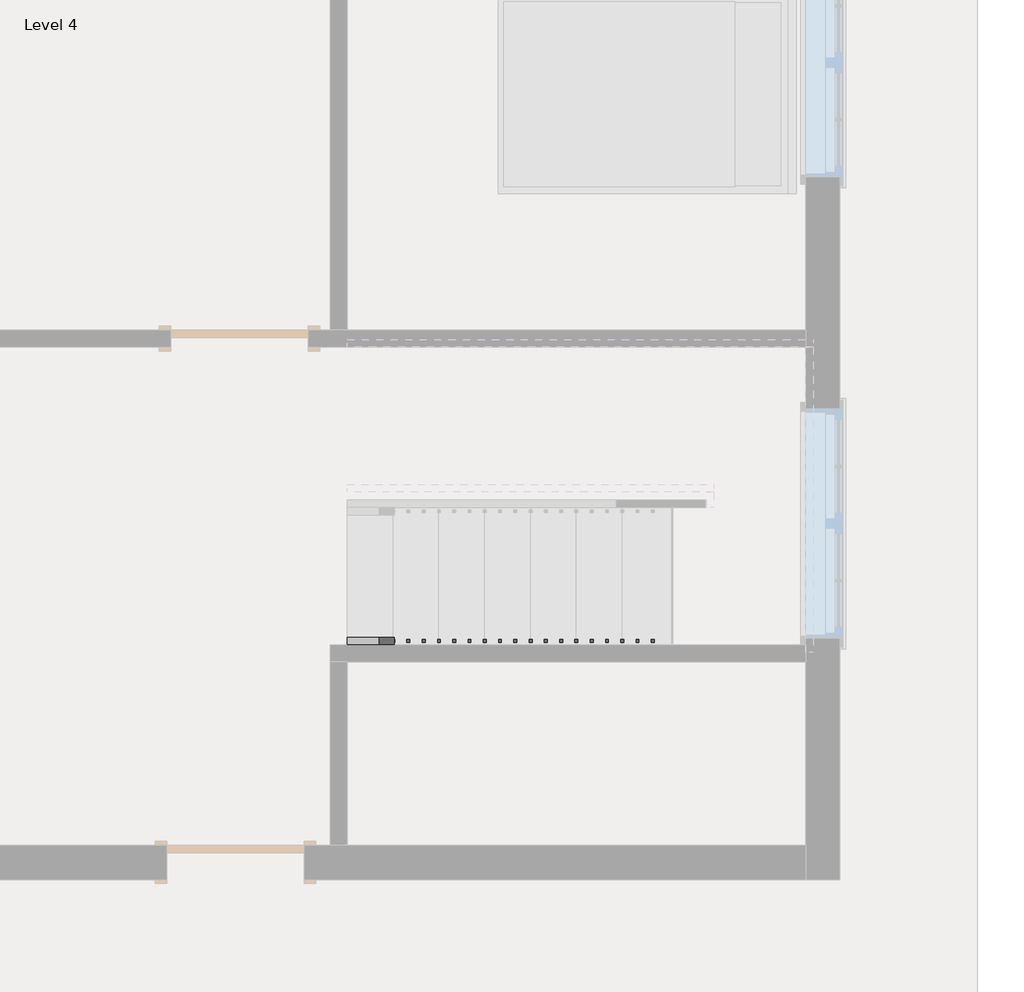
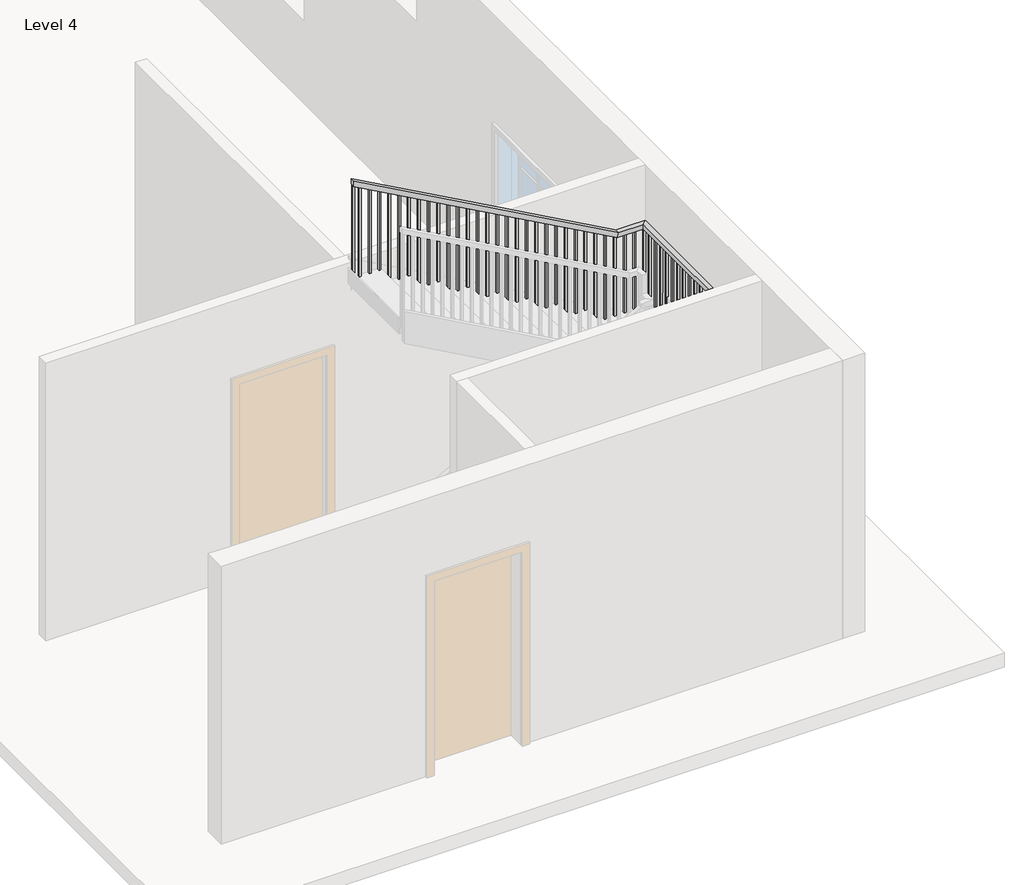
# One storey, part 2 of 3: 1 railing.
"""IFC4 building model written with IfcOpenShell, lengths in millimetres."""

from ifc_helpers import new_model, si_unit, frame, origin, place, context, project, spatial, polyline, outline, extrude, faceted_brep, element, save

model = new_model("IFC4")

# Units and contexts
model_context = context("Model", 3, world=origin())
ifc_project = project(units=[si_unit("LENGTHUNIT", "METRE", prefix="MILLI")], contexts=[model_context])

# Site, building, storey
site = spatial("IfcSite", under=ifc_project)
building = spatial("IfcBuilding", under=site)
storey = spatial("IfcBuildingStorey", under=building, Name="Level 4", Elevation=9448.8)

# Railing
placement = place(None, origin())
element("IfcRailing", 1, ObjectType="Handrail - Rectangular", at=placement, inside=storey, context=model_context, shape_type="SolidModel", body=[
    faceted_brep([(-1197.97188, -4765.70869, 10532.5333333), (-1197.97188, -4765.70869, 10474.420221), (-1197.97188, -4816.50869, 10474.420221), (-1197.97188, -4816.50869, 10532.5333333), (1240.42812, -4765.70869, 11887.2), (1253.5917222, -4765.70869, 11836.4), (1253.5917222, -4816.50869, 11836.4), (1240.42812, -4816.50869, 11887.2), (1799.22812, -4765.70869, 11887.2), (1799.22812, -4765.70869, 11836.4), (1850.02812, -4816.50869, 11836.4), (1850.02812, -4816.50869, 11887.2), (1799.22812, -2886.10869, 11887.2), (1799.22812, -2886.10869, 11836.4), (1850.02812, -2835.30869, 11836.4), (1850.02812, -2835.30869, 11887.2), (1545.22812, -2886.10869, 11887.2), (1532.0645177, -2886.10869, 11836.4), (1532.0645177, -2835.30869, 11836.4), (1545.22812, -2835.30869, 11887.2), (-1197.97188, -2886.10869, 13411.2), (-1197.97188, -2835.30869, 13411.2), (-1197.97188, -2835.30869, 13353.0868876), (-1197.97188, -2886.10869, 13353.0868876)], [[[0, 1, 2, 3]], [[1, 0, 4, 5]], [[2, 1, 5, 6]], [[3, 2, 6, 7]], [[0, 3, 7, 4]], [[5, 4, 8, 9]], [[6, 5, 9, 10]], [[7, 6, 10, 11]], [[4, 7, 11, 8]], [[9, 8, 12, 13]], [[10, 9, 13, 14]], [[11, 10, 14, 15]], [[8, 11, 15, 12]], [[13, 12, 16, 17]], [[14, 13, 17, 18]], [[15, 14, 18, 19]], [[12, 15, 19, 16]], [[20, 21, 22, 23]], [[17, 16, 20, 23]], [[18, 17, 23, 22]], [[19, 18, 22, 21]], [[16, 19, 21, 20]]]),
    extrude(outline(polyline([(13305.4618876, -1112.24688), (13316.045221, -1131.29688), (12327.4666667, -1131.29688), (12327.4666667, -1112.24688), (13305.4618876, -1112.24688)])), frame((0.0, -2870.23369, 0.0), z_axis=(0.0, 1.0, 0.0), x_axis=(0.0, 0.0, 1.0)), (0.0, 0.0, 1.0), 19.05),
    extrude(outline(polyline([(13249.0174432, -1010.64688), (13259.6007765, -1029.69688), (12327.4666667, -1029.69688), (12327.4666667, -1010.64688), (13249.0174432, -1010.64688)])), frame((0.0, -2870.23369, 0.0), z_axis=(0.0, 1.0, 0.0), x_axis=(0.0, 0.0, 1.0)), (0.0, 0.0, 1.0), 19.05),
    extrude(outline(polyline([(13192.5729988, -909.04688), (13203.1563321, -928.09688), (12327.4666667, -928.09688), (12327.4666667, -909.04688), (13192.5729988, -909.04688)])), frame((0.0, -2870.23369, 0.0), z_axis=(0.0, 1.0, 0.0), x_axis=(0.0, 0.0, 1.0)), (0.0, 0.0, 1.0), 19.05),
    extrude(outline(polyline([(13136.1285543, -807.44688), (13146.7118876, -826.49688), (12158.1333333, -826.49688), (12158.1333333, -807.44688), (13136.1285543, -807.44688)])), frame((0.0, -2870.23369, 0.0), z_axis=(0.0, 1.0, 0.0), x_axis=(0.0, 0.0, 1.0)), (0.0, 0.0, 1.0), 19.05),
    extrude(outline(polyline([(13079.6841099, -705.84688), (13090.2674432, -724.89688), (12158.1333333, -724.89688), (12158.1333333, -705.84688), (13079.6841099, -705.84688)])), frame((0.0, -2870.23369, 0.0), z_axis=(0.0, 1.0, 0.0), x_axis=(0.0, 0.0, 1.0)), (0.0, 0.0, 1.0), 19.05),
    extrude(outline(polyline([(13023.2396654, -604.24688), (13033.8229988, -623.29688), (12158.1333333, -623.29688), (12158.1333333, -604.24688), (13023.2396654, -604.24688)])), frame((0.0, -2870.23369, 0.0), z_axis=(0.0, 1.0, 0.0), x_axis=(0.0, 0.0, 1.0)), (0.0, 0.0, 1.0), 19.05),
    extrude(outline(polyline([(12966.795221, -502.64688), (12977.3785543, -521.69688), (11988.8, -521.69688), (11988.8, -502.64688), (12966.795221, -502.64688)])), frame((0.0, -2870.23369, 0.0), z_axis=(0.0, 1.0, 0.0), x_axis=(0.0, 0.0, 1.0)), (0.0, 0.0, 1.0), 19.05),
    extrude(outline(polyline([(12910.3507765, -401.04688), (12920.9341099, -420.09688), (11988.8, -420.09688), (11988.8, -401.04688), (12910.3507765, -401.04688)])), frame((0.0, -2870.23369, 0.0), z_axis=(0.0, 1.0, 0.0), x_axis=(0.0, 0.0, 1.0)), (0.0, 0.0, 1.0), 19.05),
    extrude(outline(polyline([(12853.9063321, -299.44688), (12864.4896654, -318.49688), (11988.8, -318.49688), (11988.8, -299.44688), (12853.9063321, -299.44688)])), frame((0.0, -2870.23369, 0.0), z_axis=(0.0, 1.0, 0.0), x_axis=(0.0, 0.0, 1.0)), (0.0, 0.0, 1.0), 19.05),
    extrude(outline(polyline([(12797.4618876, -197.84688), (12808.045221, -216.89688), (11819.4666667, -216.89688), (11819.4666667, -197.84688), (12797.4618876, -197.84688)])), frame((0.0, -2870.23369, 0.0), z_axis=(0.0, 1.0, 0.0), x_axis=(0.0, 0.0, 1.0)), (0.0, 0.0, 1.0), 19.05),
    extrude(outline(polyline([(12741.0174432, -96.24688), (12751.6007765, -115.29688), (11819.4666667, -115.29688), (11819.4666667, -96.24688), (12741.0174432, -96.24688)])), frame((0.0, -2870.23369, 0.0), z_axis=(0.0, 1.0, 0.0), x_axis=(0.0, 0.0, 1.0)), (0.0, 0.0, 1.0), 19.05),
    extrude(outline(polyline([(12684.5729988, 5.35312), (12695.1563321, -13.69688), (11819.4666667, -13.69688), (11819.4666667, 5.35312), (12684.5729988, 5.35312)])), frame((0.0, -2870.23369, 0.0), z_axis=(0.0, 1.0, 0.0), x_axis=(0.0, 0.0, 1.0)), (0.0, 0.0, 1.0), 19.05),
    extrude(outline(polyline([(12628.1285543, 106.95312), (12638.7118876, 87.90312), (11650.1333333, 87.90312), (11650.1333333, 106.95312), (12628.1285543, 106.95312)])), frame((0.0, -2870.23369, 0.0), z_axis=(0.0, 1.0, 0.0), x_axis=(0.0, 0.0, 1.0)), (0.0, 0.0, 1.0), 19.05),
    extrude(outline(polyline([(12571.6841099, 208.55312), (12582.2674432, 189.50312), (11650.1333333, 189.50312), (11650.1333333, 208.55312), (12571.6841099, 208.55312)])), frame((0.0, -2870.23369, 0.0), z_axis=(0.0, 1.0, 0.0), x_axis=(0.0, 0.0, 1.0)), (0.0, 0.0, 1.0), 19.05),
    extrude(outline(polyline([(12515.2396654, 310.15312), (12525.8229988, 291.10312), (11650.1333333, 291.10312), (11650.1333333, 310.15312), (12515.2396654, 310.15312)])), frame((0.0, -2870.23369, 0.0), z_axis=(0.0, 1.0, 0.0), x_axis=(0.0, 0.0, 1.0)), (0.0, 0.0, 1.0), 19.05),
    extrude(outline(polyline([(12458.795221, 411.75312), (12469.3785543, 392.70312), (11480.8, 392.70312), (11480.8, 411.75312), (12458.795221, 411.75312)])), frame((0.0, -2870.23369, 0.0), z_axis=(0.0, 1.0, 0.0), x_axis=(0.0, 0.0, 1.0)), (0.0, 0.0, 1.0), 19.05),
    extrude(outline(polyline([(12402.3507765, 513.35312), (12412.9341099, 494.30312), (11480.8, 494.30312), (11480.8, 513.35312), (12402.3507765, 513.35312)])), frame((0.0, -2870.23369, 0.0), z_axis=(0.0, 1.0, 0.0), x_axis=(0.0, 0.0, 1.0)), (0.0, 0.0, 1.0), 19.05),
    extrude(outline(polyline([(12345.9063321, 614.95312), (12356.4896654, 595.90312), (11480.8, 595.90312), (11480.8, 614.95312), (12345.9063321, 614.95312)])), frame((0.0, -2870.23369, 0.0), z_axis=(0.0, 1.0, 0.0), x_axis=(0.0, 0.0, 1.0)), (0.0, 0.0, 1.0), 19.05),
    extrude(outline(polyline([(12289.4618876, 716.55312), (12300.045221, 697.50312), (11311.4666667, 697.50312), (11311.4666667, 716.55312), (12289.4618876, 716.55312)])), frame((0.0, -2870.23369, 0.0), z_axis=(0.0, 1.0, 0.0), x_axis=(0.0, 0.0, 1.0)), (0.0, 0.0, 1.0), 19.05),
    extrude(outline(polyline([(12233.0174432, 818.15312), (12243.6007765, 799.10312), (11311.4666667, 799.10312), (11311.4666667, 818.15312), (12233.0174432, 818.15312)])), frame((0.0, -2870.23369, 0.0), z_axis=(0.0, 1.0, 0.0), x_axis=(0.0, 0.0, 1.0)), (0.0, 0.0, 1.0), 19.05),
    extrude(outline(polyline([(12176.5729988, 919.75312), (12187.1563321, 900.70312), (11311.4666667, 900.70312), (11311.4666667, 919.75312), (12176.5729988, 919.75312)])), frame((0.0, -2870.23369, 0.0), z_axis=(0.0, 1.0, 0.0), x_axis=(0.0, 0.0, 1.0)), (0.0, 0.0, 1.0), 19.05),
    extrude(outline(polyline([(12120.1285543, 1021.35312), (12130.7118876, 1002.30312), (11142.1333333, 1002.30312), (11142.1333333, 1021.35312), (12120.1285543, 1021.35312)])), frame((0.0, -2870.23369, 0.0), z_axis=(0.0, 1.0, 0.0), x_axis=(0.0, 0.0, 1.0)), (0.0, 0.0, 1.0), 19.05),
    extrude(outline(polyline([(12063.6841099, 1122.95312), (12074.2674432, 1103.90312), (11142.1333333, 1103.90312), (11142.1333333, 1122.95312), (12063.6841099, 1122.95312)])), frame((0.0, -2870.23369, 0.0), z_axis=(0.0, 1.0, 0.0), x_axis=(0.0, 0.0, 1.0)), (0.0, 0.0, 1.0), 19.05),
    extrude(outline(polyline([(12007.2396654, 1224.55312), (12017.8229988, 1205.50312), (11142.1333333, 1205.50312), (11142.1333333, 1224.55312), (12007.2396654, 1224.55312)])), frame((0.0, -2870.23369, 0.0), z_axis=(0.0, 1.0, 0.0), x_axis=(0.0, 0.0, 1.0)), (0.0, 0.0, 1.0), 19.05),
    extrude(outline(polyline([(11950.795221, 1326.15312), (11961.3785543, 1307.10312), (10972.8, 1307.10312), (10972.8, 1326.15312), (11950.795221, 1326.15312)])), frame((0.0, -2870.23369, 0.0), z_axis=(0.0, 1.0, 0.0), x_axis=(0.0, 0.0, 1.0)), (0.0, 0.0, 1.0), 19.05),
    extrude(outline(polyline([(11894.3507765, 1427.75312), (11904.9341099, 1408.70312), (10972.8, 1408.70312), (10972.8, 1427.75312), (11894.3507765, 1427.75312)])), frame((0.0, -2870.23369, 0.0), z_axis=(0.0, 1.0, 0.0), x_axis=(0.0, 0.0, 1.0)), (0.0, 0.0, 1.0), 19.05),
    extrude(outline(polyline([(11837.9063321, 1529.35312), (11848.4896654, 1510.30312), (10972.8, 1510.30312), (10972.8, 1529.35312), (11837.9063321, 1529.35312)])), frame((0.0, -2870.23369, 0.0), z_axis=(0.0, 1.0, 0.0), x_axis=(0.0, 0.0, 1.0)), (0.0, 0.0, 1.0), 19.05),
    extrude(outline(polyline([(1630.95312, -2851.18369), (1630.95312, -2870.23369), (1611.90312, -2870.23369), (1611.90312, -2851.18369), (1630.95312, -2851.18369)])), frame((0.0, 0.0, 10972.8), z_axis=(0.0, 0.0, 1.0), x_axis=(1.0, 0.0, 0.0)), (0.0, 0.0, 1.0), 863.6),
    extrude(outline(polyline([(1732.55312, -2851.18369), (1732.55312, -2870.23369), (1713.50312, -2870.23369), (1713.50312, -2851.18369), (1732.55312, -2851.18369)])), frame((0.0, 0.0, 10972.8), z_axis=(0.0, 0.0, 1.0), x_axis=(1.0, 0.0, 0.0)), (0.0, 0.0, 1.0), 863.6),
    extrude(outline(polyline([(1834.15312, -2971.83369), (1815.10312, -2971.83369), (1815.10312, -2952.78369), (1834.15312, -2952.78369), (1834.15312, -2971.83369)])), frame((0.0, 0.0, 10972.8), z_axis=(0.0, 0.0, 1.0), x_axis=(1.0, 0.0, 0.0)), (0.0, 0.0, 1.0), 863.6),
    extrude(outline(polyline([(1834.15312, -3073.43369), (1815.10312, -3073.43369), (1815.10312, -3054.38369), (1834.15312, -3054.38369), (1834.15312, -3073.43369)])), frame((0.0, 0.0, 10972.8), z_axis=(0.0, 0.0, 1.0), x_axis=(1.0, 0.0, 0.0)), (0.0, 0.0, 1.0), 863.6),
    extrude(outline(polyline([(1834.15312, -3175.03369), (1815.10312, -3175.03369), (1815.10312, -3155.98369), (1834.15312, -3155.98369), (1834.15312, -3175.03369)])), frame((0.0, 0.0, 10972.8), z_axis=(0.0, 0.0, 1.0), x_axis=(1.0, 0.0, 0.0)), (0.0, 0.0, 1.0), 863.6),
    extrude(outline(polyline([(1834.15312, -3276.63369), (1815.10312, -3276.63369), (1815.10312, -3257.58369), (1834.15312, -3257.58369), (1834.15312, -3276.63369)])), frame((0.0, 0.0, 10972.8), z_axis=(0.0, 0.0, 1.0), x_axis=(1.0, 0.0, 0.0)), (0.0, 0.0, 1.0), 863.6),
    extrude(outline(polyline([(1834.15312, -3378.23369), (1815.10312, -3378.23369), (1815.10312, -3359.18369), (1834.15312, -3359.18369), (1834.15312, -3378.23369)])), frame((0.0, 0.0, 10972.8), z_axis=(0.0, 0.0, 1.0), x_axis=(1.0, 0.0, 0.0)), (0.0, 0.0, 1.0), 863.6),
    extrude(outline(polyline([(1834.15312, -3479.83369), (1815.10312, -3479.83369), (1815.10312, -3460.78369), (1834.15312, -3460.78369), (1834.15312, -3479.83369)])), frame((0.0, 0.0, 10972.8), z_axis=(0.0, 0.0, 1.0), x_axis=(1.0, 0.0, 0.0)), (0.0, 0.0, 1.0), 863.6),
    extrude(outline(polyline([(1834.15312, -3581.43369), (1815.10312, -3581.43369), (1815.10312, -3562.38369), (1834.15312, -3562.38369), (1834.15312, -3581.43369)])), frame((0.0, 0.0, 10972.8), z_axis=(0.0, 0.0, 1.0), x_axis=(1.0, 0.0, 0.0)), (0.0, 0.0, 1.0), 863.6),
    extrude(outline(polyline([(1834.15312, -3683.03369), (1815.10312, -3683.03369), (1815.10312, -3663.98369), (1834.15312, -3663.98369), (1834.15312, -3683.03369)])), frame((0.0, 0.0, 10972.8), z_axis=(0.0, 0.0, 1.0), x_axis=(1.0, 0.0, 0.0)), (0.0, 0.0, 1.0), 863.6),
    extrude(outline(polyline([(1834.15312, -3784.63369), (1815.10312, -3784.63369), (1815.10312, -3765.58369), (1834.15312, -3765.58369), (1834.15312, -3784.63369)])), frame((0.0, 0.0, 10972.8), z_axis=(0.0, 0.0, 1.0), x_axis=(1.0, 0.0, 0.0)), (0.0, 0.0, 1.0), 863.6),
    extrude(outline(polyline([(1834.15312, -3886.23369), (1815.10312, -3886.23369), (1815.10312, -3867.18369), (1834.15312, -3867.18369), (1834.15312, -3886.23369)])), frame((0.0, 0.0, 10972.8), z_axis=(0.0, 0.0, 1.0), x_axis=(1.0, 0.0, 0.0)), (0.0, 0.0, 1.0), 863.6),
    extrude(outline(polyline([(1834.15312, -3987.83369), (1815.10312, -3987.83369), (1815.10312, -3968.78369), (1834.15312, -3968.78369), (1834.15312, -3987.83369)])), frame((0.0, 0.0, 10972.8), z_axis=(0.0, 0.0, 1.0), x_axis=(1.0, 0.0, 0.0)), (0.0, 0.0, 1.0), 863.6),
    extrude(outline(polyline([(1834.15312, -4089.43369), (1815.10312, -4089.43369), (1815.10312, -4070.38369), (1834.15312, -4070.38369), (1834.15312, -4089.43369)])), frame((0.0, 0.0, 10972.8), z_axis=(0.0, 0.0, 1.0), x_axis=(1.0, 0.0, 0.0)), (0.0, 0.0, 1.0), 863.6),
    extrude(outline(polyline([(1834.15312, -4191.03369), (1815.10312, -4191.03369), (1815.10312, -4171.98369), (1834.15312, -4171.98369), (1834.15312, -4191.03369)])), frame((0.0, 0.0, 10972.8), z_axis=(0.0, 0.0, 1.0), x_axis=(1.0, 0.0, 0.0)), (0.0, 0.0, 1.0), 863.6),
    extrude(outline(polyline([(1834.15312, -4292.63369), (1815.10312, -4292.63369), (1815.10312, -4273.58369), (1834.15312, -4273.58369), (1834.15312, -4292.63369)])), frame((0.0, 0.0, 10972.8), z_axis=(0.0, 0.0, 1.0), x_axis=(1.0, 0.0, 0.0)), (0.0, 0.0, 1.0), 863.6),
    extrude(outline(polyline([(1834.15312, -4394.23369), (1815.10312, -4394.23369), (1815.10312, -4375.18369), (1834.15312, -4375.18369), (1834.15312, -4394.23369)])), frame((0.0, 0.0, 10972.8), z_axis=(0.0, 0.0, 1.0), x_axis=(1.0, 0.0, 0.0)), (0.0, 0.0, 1.0), 863.6),
    extrude(outline(polyline([(1834.15312, -4495.83369), (1815.10312, -4495.83369), (1815.10312, -4476.78369), (1834.15312, -4476.78369), (1834.15312, -4495.83369)])), frame((0.0, 0.0, 10972.8), z_axis=(0.0, 0.0, 1.0), x_axis=(1.0, 0.0, 0.0)), (0.0, 0.0, 1.0), 863.6),
    extrude(outline(polyline([(1834.15312, -4597.43369), (1815.10312, -4597.43369), (1815.10312, -4578.38369), (1834.15312, -4578.38369), (1834.15312, -4597.43369)])), frame((0.0, 0.0, 10972.8), z_axis=(0.0, 0.0, 1.0), x_axis=(1.0, 0.0, 0.0)), (0.0, 0.0, 1.0), 863.6),
    extrude(outline(polyline([(1834.15312, -4699.03369), (1815.10312, -4699.03369), (1815.10312, -4679.98369), (1834.15312, -4679.98369), (1834.15312, -4699.03369)])), frame((0.0, 0.0, 10972.8), z_axis=(0.0, 0.0, 1.0), x_axis=(1.0, 0.0, 0.0)), (0.0, 0.0, 1.0), 863.6),
    extrude(outline(polyline([(1738.90312, -4800.63369), (1738.90312, -4781.58369), (1757.95312, -4781.58369), (1757.95312, -4800.63369), (1738.90312, -4800.63369)])), frame((0.0, 0.0, 10972.8), z_axis=(0.0, 0.0, 1.0), x_axis=(1.0, 0.0, 0.0)), (0.0, 0.0, 1.0), 863.6),
    extrude(outline(polyline([(1637.30312, -4800.63369), (1637.30312, -4781.58369), (1656.35312, -4781.58369), (1656.35312, -4800.63369), (1637.30312, -4800.63369)])), frame((0.0, 0.0, 10972.8), z_axis=(0.0, 0.0, 1.0), x_axis=(1.0, 0.0, 0.0)), (0.0, 0.0, 1.0), 863.6),
    extrude(outline(polyline([(1535.70312, -4800.63369), (1535.70312, -4781.58369), (1554.75312, -4781.58369), (1554.75312, -4800.63369), (1535.70312, -4800.63369)])), frame((0.0, 0.0, 10972.8), z_axis=(0.0, 0.0, 1.0), x_axis=(1.0, 0.0, 0.0)), (0.0, 0.0, 1.0), 863.6),
    extrude(outline(polyline([(1434.10312, -4800.63369), (1434.10312, -4781.58369), (1453.15312, -4781.58369), (1453.15312, -4800.63369), (1434.10312, -4800.63369)])), frame((0.0, 0.0, 10972.8), z_axis=(0.0, 0.0, 1.0), x_axis=(1.0, 0.0, 0.0)), (0.0, 0.0, 1.0), 863.6),
    extrude(outline(polyline([(1332.50312, -4800.63369), (1332.50312, -4781.58369), (1351.55312, -4781.58369), (1351.55312, -4800.63369), (1332.50312, -4800.63369)])), frame((0.0, 0.0, 10972.8), z_axis=(0.0, 0.0, 1.0), x_axis=(1.0, 0.0, 0.0)), (0.0, 0.0, 1.0), 863.6),
    extrude(outline(polyline([(11834.3785543, 1249.95312), (11823.795221, 1230.90312), (10972.8, 1230.90312), (10972.8, 1249.95312), (11834.3785543, 1249.95312)])), frame((0.0, -4800.63369, 0.0), z_axis=(0.0, 1.0, 0.0), x_axis=(0.0, 0.0, 1.0)), (0.0, 0.0, 1.0), 19.05),
    extrude(outline(polyline([(11777.9341099, 1148.35312), (11767.3507765, 1129.30312), (10803.4666667, 1129.30312), (10803.4666667, 1148.35312), (11777.9341099, 1148.35312)])), frame((0.0, -4800.63369, 0.0), z_axis=(0.0, 1.0, 0.0), x_axis=(0.0, 0.0, 1.0)), (0.0, 0.0, 1.0), 19.05),
    extrude(outline(polyline([(11721.4896654, 1046.75312), (11710.9063321, 1027.70312), (10803.4666667, 1027.70312), (10803.4666667, 1046.75312), (11721.4896654, 1046.75312)])), frame((0.0, -4800.63369, 0.0), z_axis=(0.0, 1.0, 0.0), x_axis=(0.0, 0.0, 1.0)), (0.0, 0.0, 1.0), 19.05),
    extrude(outline(polyline([(11665.045221, 945.15312), (11654.4618876, 926.10312), (10803.4666667, 926.10312), (10803.4666667, 945.15312), (11665.045221, 945.15312)])), frame((0.0, -4800.63369, 0.0), z_axis=(0.0, 1.0, 0.0), x_axis=(0.0, 0.0, 1.0)), (0.0, 0.0, 1.0), 19.05),
    extrude(outline(polyline([(11608.6007765, 843.55312), (11598.0174432, 824.50312), (10634.1333333, 824.50312), (10634.1333333, 843.55312), (11608.6007765, 843.55312)])), frame((0.0, -4800.63369, 0.0), z_axis=(0.0, 1.0, 0.0), x_axis=(0.0, 0.0, 1.0)), (0.0, 0.0, 1.0), 19.05),
    extrude(outline(polyline([(11552.1563321, 741.95312), (11541.5729988, 722.90312), (10634.1333333, 722.90312), (10634.1333333, 741.95312), (11552.1563321, 741.95312)])), frame((0.0, -4800.63369, 0.0), z_axis=(0.0, 1.0, 0.0), x_axis=(0.0, 0.0, 1.0)), (0.0, 0.0, 1.0), 19.05),
    extrude(outline(polyline([(11495.7118876, 640.35312), (11485.1285543, 621.30312), (10634.1333333, 621.30312), (10634.1333333, 640.35312), (11495.7118876, 640.35312)])), frame((0.0, -4800.63369, 0.0), z_axis=(0.0, 1.0, 0.0), x_axis=(0.0, 0.0, 1.0)), (0.0, 0.0, 1.0), 19.05),
    extrude(outline(polyline([(11439.2674432, 538.75312), (11428.6841099, 519.70312), (10464.8, 519.70312), (10464.8, 538.75312), (11439.2674432, 538.75312)])), frame((0.0, -4800.63369, 0.0), z_axis=(0.0, 1.0, 0.0), x_axis=(0.0, 0.0, 1.0)), (0.0, 0.0, 1.0), 19.05),
    extrude(outline(polyline([(11382.8229988, 437.15312), (11372.2396654, 418.10312), (10464.8, 418.10312), (10464.8, 437.15312), (11382.8229988, 437.15312)])), frame((0.0, -4800.63369, 0.0), z_axis=(0.0, 1.0, 0.0), x_axis=(0.0, 0.0, 1.0)), (0.0, 0.0, 1.0), 19.05),
    extrude(outline(polyline([(11326.3785543, 335.55312), (11315.795221, 316.50312), (10464.8, 316.50312), (10464.8, 335.55312), (11326.3785543, 335.55312)])), frame((0.0, -4800.63369, 0.0), z_axis=(0.0, 1.0, 0.0), x_axis=(0.0, 0.0, 1.0)), (0.0, 0.0, 1.0), 19.05),
    extrude(outline(polyline([(11269.9341099, 233.95312), (11259.3507765, 214.90312), (10295.4666667, 214.90312), (10295.4666667, 233.95312), (11269.9341099, 233.95312)])), frame((0.0, -4800.63369, 0.0), z_axis=(0.0, 1.0, 0.0), x_axis=(0.0, 0.0, 1.0)), (0.0, 0.0, 1.0), 19.05),
    extrude(outline(polyline([(11213.4896654, 132.35312), (11202.9063321, 113.30312), (10295.4666667, 113.30312), (10295.4666667, 132.35312), (11213.4896654, 132.35312)])), frame((0.0, -4800.63369, 0.0), z_axis=(0.0, 1.0, 0.0), x_axis=(0.0, 0.0, 1.0)), (0.0, 0.0, 1.0), 19.05),
    extrude(outline(polyline([(11157.045221, 30.75312), (11146.4618876, 11.70312), (10295.4666667, 11.70312), (10295.4666667, 30.75312), (11157.045221, 30.75312)])), frame((0.0, -4800.63369, 0.0), z_axis=(0.0, 1.0, 0.0), x_axis=(0.0, 0.0, 1.0)), (0.0, 0.0, 1.0), 19.05),
    extrude(outline(polyline([(11100.6007765, -70.84688), (11090.0174432, -89.89688), (10126.1333333, -89.89688), (10126.1333333, -70.84688), (11100.6007765, -70.84688)])), frame((0.0, -4800.63369, 0.0), z_axis=(0.0, 1.0, 0.0), x_axis=(0.0, 0.0, 1.0)), (0.0, 0.0, 1.0), 19.05),
    extrude(outline(polyline([(11044.1563321, -172.44688), (11033.5729988, -191.49688), (10126.1333333, -191.49688), (10126.1333333, -172.44688), (11044.1563321, -172.44688)])), frame((0.0, -4800.63369, 0.0), z_axis=(0.0, 1.0, 0.0), x_axis=(0.0, 0.0, 1.0)), (0.0, 0.0, 1.0), 19.05),
    extrude(outline(polyline([(10987.7118876, -274.04688), (10977.1285543, -293.09688), (10126.1333333, -293.09688), (10126.1333333, -274.04688), (10987.7118876, -274.04688)])), frame((0.0, -4800.63369, 0.0), z_axis=(0.0, 1.0, 0.0), x_axis=(0.0, 0.0, 1.0)), (0.0, 0.0, 1.0), 19.05),
    extrude(outline(polyline([(10931.2674432, -375.64688), (10920.6841099, -394.69688), (9956.8, -394.69688), (9956.8, -375.64688), (10931.2674432, -375.64688)])), frame((0.0, -4800.63369, 0.0), z_axis=(0.0, 1.0, 0.0), x_axis=(0.0, 0.0, 1.0)), (0.0, 0.0, 1.0), 19.05),
    extrude(outline(polyline([(10874.8229988, -477.24688), (10864.2396654, -496.29688), (9956.8, -496.29688), (9956.8, -477.24688), (10874.8229988, -477.24688)])), frame((0.0, -4800.63369, 0.0), z_axis=(0.0, 1.0, 0.0), x_axis=(0.0, 0.0, 1.0)), (0.0, 0.0, 1.0), 19.05),
    extrude(outline(polyline([(10818.3785543, -578.84688), (10807.795221, -597.89688), (9956.8, -597.89688), (9956.8, -578.84688), (10818.3785543, -578.84688)])), frame((0.0, -4800.63369, 0.0), z_axis=(0.0, 1.0, 0.0), x_axis=(0.0, 0.0, 1.0)), (0.0, 0.0, 1.0), 19.05),
    extrude(outline(polyline([(10761.9341099, -680.44688), (10751.3507765, -699.49688), (9787.4666667, -699.49688), (9787.4666667, -680.44688), (10761.9341099, -680.44688)])), frame((0.0, -4800.63369, 0.0), z_axis=(0.0, 1.0, 0.0), x_axis=(0.0, 0.0, 1.0)), (0.0, 0.0, 1.0), 19.05),
    extrude(outline(polyline([(10705.4896654, -782.04688), (10694.9063321, -801.09688), (9787.4666667, -801.09688), (9787.4666667, -782.04688), (10705.4896654, -782.04688)])), frame((0.0, -4800.63369, 0.0), z_axis=(0.0, 1.0, 0.0), x_axis=(0.0, 0.0, 1.0)), (0.0, 0.0, 1.0), 19.05),
    extrude(outline(polyline([(10649.045221, -883.64688), (10638.4618876, -902.69688), (9787.4666667, -902.69688), (9787.4666667, -883.64688), (10649.045221, -883.64688)])), frame((0.0, -4800.63369, 0.0), z_axis=(0.0, 1.0, 0.0), x_axis=(0.0, 0.0, 1.0)), (0.0, 0.0, 1.0), 19.05),
    extrude(outline(polyline([(10592.6007765, -985.24688), (10582.0174432, -1004.29688), (9618.1333333, -1004.29688), (9618.1333333, -985.24688), (10592.6007765, -985.24688)])), frame((0.0, -4800.63369, 0.0), z_axis=(0.0, 1.0, 0.0), x_axis=(0.0, 0.0, 1.0)), (0.0, 0.0, 1.0), 19.05),
    extrude(outline(polyline([(10536.1563321, -1086.84688), (10525.5729988, -1105.89688), (9618.1333333, -1105.89688), (9618.1333333, -1086.84688), (10536.1563321, -1086.84688)])), frame((0.0, -4800.63369, 0.0), z_axis=(0.0, 1.0, 0.0), x_axis=(0.0, 0.0, 1.0)), (0.0, 0.0, 1.0), 19.05),
    extrude(outline(polyline([(1834.15312, -2870.23369), (1815.10312, -2870.23369), (1815.10312, -2851.18369), (1834.15312, -2851.18369), (1834.15312, -2870.23369)])), frame((0.0, 0.0, 10972.8), z_axis=(0.0, 0.0, 1.0), x_axis=(1.0, 0.0, 0.0)), (0.0, 0.0, 1.0), 863.6),
    extrude(outline(polyline([(1815.10312, -4800.63369), (1815.10312, -4781.58369), (1834.15312, -4781.58369), (1834.15312, -4800.63369), (1815.10312, -4800.63369)])), frame((0.0, 0.0, 10972.8), z_axis=(0.0, 0.0, 1.0), x_axis=(1.0, 0.0, 0.0)), (0.0, 0.0, 1.0), 863.6),
    extrude(outline(polyline([(13342.5035543, -1178.92188), (13353.0868876, -1197.97188), (12327.4666667, -1197.97188), (12327.4666667, -1178.92188), (13342.5035543, -1178.92188)])), frame((0.0, -2870.23369, 0.0), z_axis=(0.0, 1.0, 0.0), x_axis=(0.0, 0.0, 1.0)), (0.0, 0.0, 1.0), 19.05),
    extrude(outline(polyline([(10485.0035543, -1178.92188), (10474.420221, -1197.97188), (9618.1333333, -1197.97188), (9618.1333333, -1178.92188), (10485.0035543, -1178.92188)])), frame((0.0, -4800.63369, 0.0), z_axis=(0.0, 1.0, 0.0), x_axis=(0.0, 0.0, 1.0)), (0.0, 0.0, 1.0), 19.05),
])

save(model, "model.ifc")

# Revit data of these elements
# Type "Handrail - Rectangular"
#   Assembly Code = "C2010400"
#   built-in parameter 1008612 = 0.0416667 (stored number, unit not read)
#   built-in parameter 1008611 = 0.0416667 (stored number, unit not read)
#   built-in parameter 1008609 = 0.333333 (stored number, unit not read)
#   built-in parameter 1008604 = 0.166667 (stored number, unit not read)
#   built-in parameter 1008603 = 0.166667 (stored number, unit not read)
#   Railing Height = 3' - 0"
#   built-in parameter 1008630 = 2
#   built-in parameter 1008610 = 2
#   built-in parameter 1008618 = Baluster - Square : 3/4"
# Element 1 (IfcRailing, "Handrail - Rectangular")
#   Phase Created = New Construction
